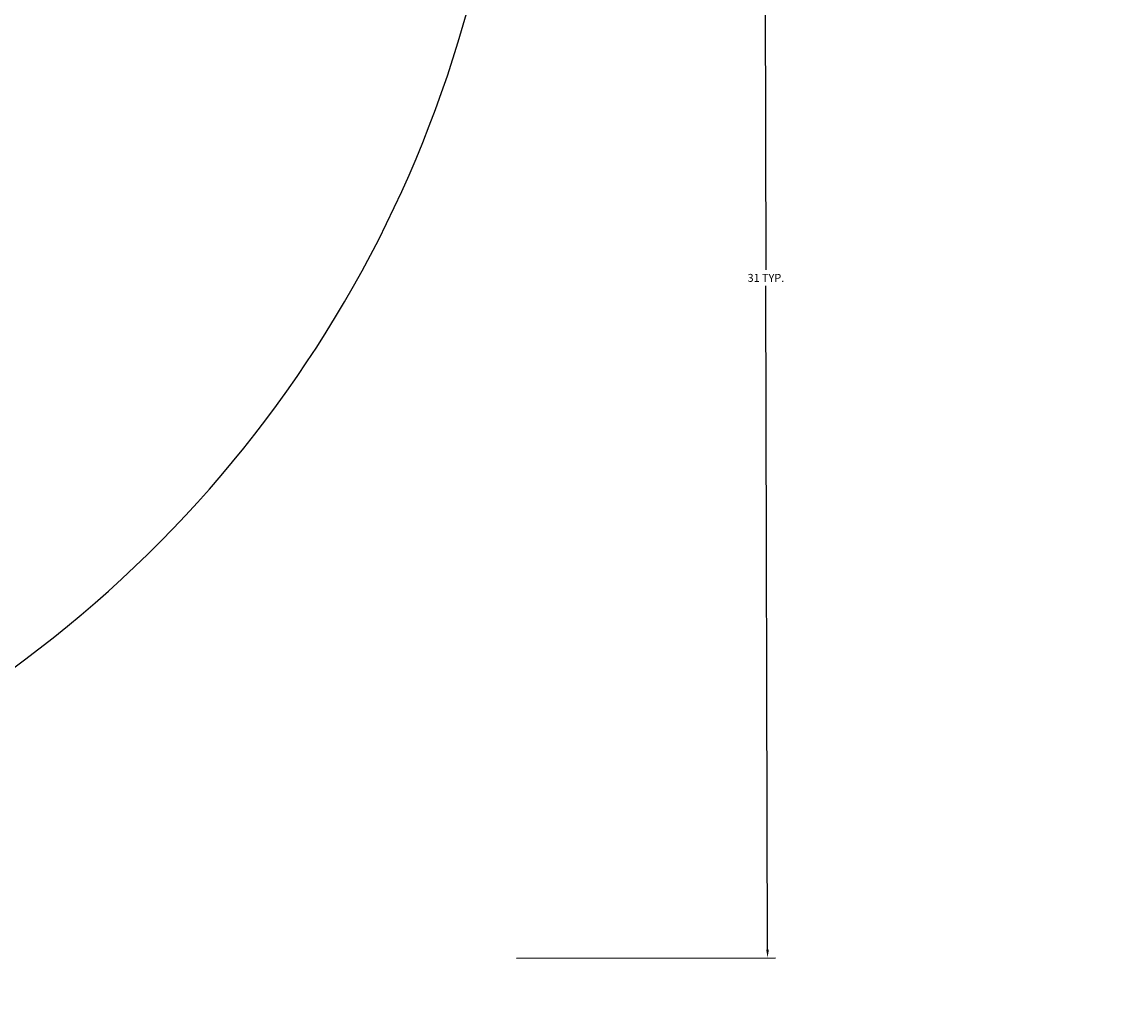
# Model space of a CAD drawing. Units: inches. Extents: x 963 to 2075, y 289 to 2657.
# Tile 10 of 98: x 1399 to 1424, y 1675 to 1696. Entities that reach past the tile are written whole.
import ezdxf

# ---------------------------------------------------------------- set-up
doc = ezdxf.new("R2010")
doc.units = ezdxf.units.IN
for name, color, linetype, lineweight in [('A-ANNO-DIMS', 2, 'Continuous', 18), ('A-DOOR', 4, 'Continuous', 25), ('A-WALL-PATT', 8, 'Continuous', 13)]:
    doc.layers.add(name, color=color, linetype=linetype, lineweight=lineweight)
doc.styles.get("Standard").update_dxf_attribs({"font": 'arial.ttf'})
doc.dimstyles.get("Standard").update_dxf_attribs({"dimtxt": 0.18, "dimasz": 0.18, "dimexe": 0.18, "dimexo": 0.0625, "dimgap": 0.09, "dimtad": 0, "dimtih": 1, "dimtoh": 1, "dimdec": 4, "dimzin": 0, "dimdsep": 46, "dimtxsty": 'Standard', "dimcen": 0.09, "dimadec": 0, "dimazin": 0, "dimtfac": 1, "dimtdec": 4, "dimtofl": 0, "dimtmove": 0, "dimatfit": 3, "dimfxl": 1, "dimtolj": 1, "dimtzin": 0, "dimarcsym": 0})

# ---------------------------------------------------------------- blocks, each defined once
blk = doc.blocks.new('DOOR-5')
blk.add_arc((27.907, 27.321), 27.321, 161.4794, 270)
blk = doc.blocks.new('*D39')
at = {"layer": 'A-ANNO-DIMS', "color": 0, "lineweight": -2, "transparency": 16777216}
for p, q in [((1410.194, 1705.998), (1416.049, 1706.012)), ((1415.869, 1705.832), (1415.906, 1690.845)), ((1415.944, 1675.494), (1415.907, 1690.481)), ((1410.269, 1675.3), (1416.124, 1675.314))]:
    blk.add_line(p, q, dxfattribs=at)
at = {"layer": 'A-ANNO-DIMS', "color": 0, "transparency": 16777216}
for points in [[(1415.899, 1705.832), (1415.839, 1705.832), (1415.869, 1706.012)], [(1415.974, 1675.494), (1415.914, 1675.494), (1415.944, 1675.314)]]:
    blk.add_solid(points, dxfattribs=at)
at = {"layer": 'Defpoints', "color": 0, "transparency": 16777216}
for p in [(1410.131, 1705.998), (1415.869, 1706.012), (1410.207, 1675.299)]:
    blk.add_point(p, dxfattribs=at)
at = {"layer": 'A-ANNO-DIMS', "color": 0, "transparency": 16777216, "insert": (1415.906, 1690.663), "char_height": 0.18, "attachment_point": 5}
blk.add_mtext('\\A1;31 TYP.', dxfattribs=at)

msp = doc.modelspace()

# ---------------------------------------------------------------- hatches: boundary and pattern name
at = {"layer": 'A-WALL-PATT'}
h = msp.add_hatch(dxfattribs=at)
h.set_pattern_fill('ANSI32', color=256)
h.paths.add_polyline_path([(1296.922, 2558.318), (1203.922, 2558.318), (1203.922, 2493.818), (1191.533, 2493.818), (1191.533, 2489.318), (1211.063, 2489.318), (1211.063, 2492.02), (1211.063, 2493.818), (1208.422, 2493.818), (1208.422, 2553.818), (1292.422, 2553.818), (1292.422, 2538.863), (1296.922, 2538.863)])
h.paths.add_polyline_path([(1442.422, 2558.318), (1349.422, 2558.318), (1349.422, 2538.943), (1353.922, 2538.943), (1353.922, 2553.818), (1437.922, 2553.818), (1437.922, 2493.818), (1434.542, 2493.818), (1434.542, 2489.318), (1448.311, 2489.318), (1448.311, 2491.568), (1448.311, 2493.818), (1442.422, 2493.818)])
h.paths.add_polyline_path([(1415.554, 2491.568), (1415.554, 2493.818), (1340.941, 2493.818), (1340.941, 2489.318), (1371.922, 2489.318), (1371.922, 2378.318), (1367.596, 2378.318), (1367.596, 2373.818), (1371.922, 2373.818), (1371.922, 2355.185), (1376.422, 2355.185), (1376.422, 2489.318), (1415.554, 2489.318)])
h.paths.add_polyline_path([(1304.941, 2491.568), (1304.941, 2493.818), (1296.922, 2493.818), (1296.922, 2514.863), (1292.422, 2514.863), (1292.422, 2493.818), (1232.808, 2493.818), (1232.808, 2489.318), (1256.422, 2489.318), (1256.422, 2327.318), (1253.714, 2327.318), (1253.714, 2322.818), (1328.422, 2322.818), (1328.422, 2331.147), (1323.922, 2331.147), (1323.922, 2327.318), (1260.922, 2327.318), (1260.922, 2373.818), (1323.922, 2373.818), (1323.922, 2357.812), (1328.422, 2357.812), (1328.422, 2373.818), (1346.007, 2373.818), (1346.007, 2376.068), (1346.007, 2378.318), (1260.922, 2378.318), (1260.922, 2489.318), (1304.941, 2489.318)])
h.paths.add_polyline_path([(1226.654, 2327.318), (1124.422, 2327.318), (1124.422, 2347.447), (1119.922, 2347.447), (1119.922, 2322.818), (1163.422, 2322.818), (1163.422, 2305.435), (1165.672, 2305.435), (1167.922, 2305.435), (1167.922, 2322.818), (1226.654, 2322.818), (1226.654, 2325.068)])
h.paths.add_polyline_path([(1095.922, 2489.318), (1124.422, 2489.318), (1131.533, 2489.318), (1131.533, 2491.568), (1131.533, 2493.818), (1119.922, 2493.818), (1091.422, 2493.818), (1091.422, 2417.318), (1095.922, 2417.318), (1119.922, 2417.318), (1119.922, 2407.447), (1124.422, 2407.447), (1124.422, 2421.818), (1095.922, 2421.818)])
h.paths.add_polyline_path([(1512.922, 2558.318), (1508.422, 2558.318), (1508.422, 2493.818), (1503.401, 2493.818), (1503.401, 2489.318), (1508.422, 2489.318), (1508.422, 2327.318), (1376.422, 2327.318), (1376.422, 2330.273), (1371.922, 2330.273), (1371.922, 2298.744), (1376.422, 2298.744), (1376.422, 2322.818), (1508.422, 2322.818), (1508.422, 2165.318), (1504.255, 2165.318), (1504.255, 2160.818), (1508.422, 2160.818), (1508.422, 2108.318), (1512.922, 2108.318), (1512.922, 2160.818), (1516.182, 2160.818), (1516.182, 2163.068), (1516.182, 2165.318), (1512.922, 2165.318), (1512.922, 2322.818), (1644.922, 2322.818), (1644.922, 2298.744), (1649.422, 2298.744), (1649.422, 2322.818), (1649.422, 2330.944), (1647.172, 2330.944), (1644.922, 2330.944), (1644.922, 2327.318), (1512.922, 2327.318), (1512.922, 2489.318), (1516.759, 2489.318), (1516.759, 2491.568), (1516.759, 2493.818), (1512.922, 2493.818)])
h.paths.add_polyline_path([(1671.922, 2558.318), (1578.922, 2558.318), (1578.922, 2493.818), (1573.526, 2493.818), (1573.526, 2489.318), (1586.537, 2489.318), (1586.537, 2491.568), (1586.537, 2493.818), (1583.422, 2493.818), (1583.422, 2553.818), (1667.422, 2553.818), (1667.422, 2541.109), (1671.922, 2541.109)])
h.paths.add_polyline_path([(1681.257, 2493.818), (1671.922, 2493.818), (1671.922, 2517.109), (1667.422, 2517.109), (1667.422, 2493.818), (1610.218, 2493.818), (1610.218, 2489.318), (1644.922, 2489.318), (1644.922, 2357.865), (1649.422, 2357.865), (1649.422, 2373.818), (1652.203, 2373.818), (1652.203, 2375.827), (1652.203, 2378.318), (1649.422, 2378.318), (1649.422, 2489.318), (1681.257, 2489.318), (1681.257, 2491.568)])
h.paths.add_polyline_path([(1821.922, 2558.318), (1728.922, 2558.318), (1728.922, 2541), (1733.422, 2541), (1733.422, 2553.818), (1817.422, 2553.818), (1817.422, 2493.818), (1813.507, 2493.818), (1813.507, 2489.318), (1830.078, 2489.318), (1830.078, 2491.568), (1830.078, 2493.818), (1821.922, 2493.818)])
h.paths.add_polyline_path([(1794.244, 2493.818), (1717.257, 2493.818), (1717.257, 2489.318), (1760.422, 2489.318), (1760.422, 2378.318), (1674.401, 2378.318), (1674.401, 2373.818), (1692.922, 2373.818), (1692.922, 2356.954), (1697.422, 2356.954), (1697.422, 2373.818), (1760.422, 2373.818), (1760.422, 2327.318), (1697.422, 2327.318), (1697.422, 2333.341), (1692.922, 2333.341), (1692.922, 2322.818), (1768.037, 2322.818), (1768.037, 2325.068), (1768.037, 2327.318), (1764.922, 2327.318), (1764.922, 2489.318), (1794.244, 2489.318)])
h.paths.add_polyline_path([(1733.422, 2517), (1728.922, 2517), (1728.922, 2493.818), (1733.422, 2493.818)], flags=17)
h.paths.add_polyline_path([(1929.922, 2493.818), (1890.078, 2493.818), (1890.078, 2489.318), (1896.922, 2489.318), (1925.422, 2489.318), (1925.422, 2421.818), (1896.922, 2421.818), (1896.922, 2408.318), (1901.422, 2408.318), (1901.422, 2417.318), (1925.422, 2417.318), (1929.922, 2417.318)])
h.paths.add_polyline_path([(1901.422, 2348.318), (1896.922, 2348.318), (1896.922, 2327.318), (1800.423, 2327.318), (1800.423, 2322.818), (1853.422, 2322.818), (1853.422, 2309.453), (1857.922, 2309.453), (1857.922, 2322.818), (1901.422, 2322.818)])
h.paths.add_polyline_path([(1857.922, 2249.453), (1853.422, 2249.453), (1853.422, 2214.818), (1686.309, 2214.818), (1686.309, 2210.318), (1853.422, 2210.318), (1853.422, 2202.134), (1857.922, 2202.134), (1857.922, 2210.318)])
h.paths.add_polyline_path([(1857.922, 2142.134), (1853.422, 2142.134), (1853.422, 2115.422), (1841.422, 2115.422), (1841.422, 2088.531), (1841.422, 2046.949), (1845.922, 2046.949), (1845.922, 2110.922), (1905.922, 2110.922), (1905.922, 2092.517), (1910.422, 2092.517), (1910.422, 2115.422), (1857.922, 2115.422)])
h.paths.add_polyline_path([(1532.436, 1482.342), (1573.456, 1482.342), (1573.456, 1501), (1532.436, 1501)], flags=9)
h.paths.add_polyline_path([(1438.658, 1486.302), (1479.678, 1486.302), (1479.678, 1504.96), (1438.658, 1504.96)], flags=9)
h.paths.add_polyline_path([(1411.215, 1365.308), (1659.139, 1365.308), (1659.139, 1402.401), (1411.215, 1402.401)], flags=9)
h.paths.add_polyline_path([(1185.671, 2296.298), (1248.16, 2296.298), (1248.16, 2314.955), (1185.671, 2314.955)], flags=9)
h.paths.add_polyline_path([(1177.31, 2187.35), (1216.15, 2187.35), (1216.15, 2206.007), (1177.31, 2206.007)], flags=9)
h.paths.add_polyline_path([(1295.101, 1602.083), (1328.26, 1602.083), (1328.26, 1620.741), (1295.101, 1620.741)], flags=9)
h.paths.add_polyline_path([(1525.126, 2005.99), (1558.39, 2005.99), (1558.39, 2024.648), (1525.126, 2024.648)], flags=9)
h.paths.add_polyline_path([(1459.606, 1977.125), (1472.195, 1977.125), (1472.195, 1987.429), (1459.606, 1987.429)], flags=9)
h.paths.add_polyline_path([(1467.815, 2053.676), (1480.018, 2053.676), (1480.018, 2063.979), (1467.815, 2063.979)], flags=9)
h.paths.add_polyline_path([(1555.184, 2119.02), (1584.563, 2119.02), (1584.563, 2137.678), (1555.184, 2137.678)], flags=25)
h.paths.add_polyline_path([(1405.389, 2115.291), (1444.478, 2115.291), (1444.478, 2133.948), (1405.389, 2133.948)], flags=25)
h.paths.add_polyline_path([(1698.482, 2004.259), (1727.695, 2004.259), (1727.695, 2022.916), (1698.482, 2022.916)], flags=9)
h.paths.add_polyline_path([(1612.158, 1972.855), (1629.016, 1972.855), (1629.016, 1983.159), (1612.158, 1983.159)], flags=9)
h.paths.add_polyline_path([(1608.289, 2060.036), (1625.147, 2060.036), (1625.147, 2070.34), (1608.289, 2070.34)], flags=9)
h.paths.add_polyline_path([(1527.954, 1684.402), (1566.795, 1684.402), (1566.795, 1703.06), (1527.954, 1703.06)], flags=9)
h.paths.add_polyline_path([(1422.792, 1683.59), (1461.633, 1683.59), (1461.633, 1702.247), (1422.792, 1702.247)], flags=9)
h.paths.add_polyline_path([(1531.262, 1732.459), (1574.015, 1732.459), (1574.015, 1751.116), (1531.262, 1751.116)], flags=9)
h.paths.add_polyline_path([(1402.872, 1732.845), (1439.799, 1732.845), (1439.799, 1751.502), (1402.872, 1751.502)], flags=9)
h.paths.add_polyline_path([(1243.122, 1923.132), (1281.962, 1923.132), (1281.962, 1941.79), (1243.122, 1941.79)], flags=9)
h.paths.add_polyline_path([(1181.752, 1792.268), (1244.241, 1792.268), (1244.241, 1810.926), (1181.752, 1810.926)], flags=9)
h.paths.add_polyline_path([(1265.822, 1670.3), (1316.071, 1670.3), (1316.071, 1688.957), (1265.822, 1688.957)], flags=9)
h.paths.add_polyline_path([(1140.263, 1676.054), (1179.104, 1676.054), (1179.104, 1694.711), (1140.263, 1694.711)], flags=9)
h.paths.add_polyline_path([(1107.49, 1490.889), (1143.374, 1490.889), (1143.374, 1509.546), (1107.49, 1509.546)], flags=9)
h.paths.add_polyline_path([(1217.584, 1483.899), (1246.741, 1483.899), (1246.741, 1502.556), (1217.584, 1502.556)], flags=9)
h.paths.add_polyline_path([(1389.21, 1486.919), (1418.367, 1486.919), (1418.367, 1505.576), (1389.21, 1505.576)], flags=9)
h.paths.add_polyline_path([(1672.208, 1602.083), (1705.366, 1602.083), (1705.366, 1620.741), (1672.208, 1620.741)], flags=9)
h.paths.add_polyline_path([(1752.082, 1522.638), (1781.24, 1522.638), (1781.24, 1541.295), (1752.082, 1541.295)], flags=9)
h.paths.add_polyline_path([(1848.275, 1491.26), (1884.158, 1491.26), (1884.158, 1509.918), (1848.275, 1509.918)], flags=9)
h.paths.add_polyline_path([(1822.47, 1685.62), (1861.31, 1685.62), (1861.31, 1704.278), (1822.47, 1704.278)], flags=9)
h.paths.add_polyline_path([(1713.195, 1672.232), (1763.444, 1672.232), (1763.444, 1690.889), (1713.195, 1690.889)], flags=9)
h.paths.add_polyline_path([(1736.619, 1790.578), (1799.109, 1790.578), (1799.109, 1809.235), (1736.619, 1809.235)], flags=9)
h.paths.add_polyline_path([(1691.491, 1916.355), (1730.332, 1916.355), (1730.332, 1935.013), (1691.491, 1935.013)], flags=9)
h.paths.add_polyline_path([(1764.872, 1973.922), (1794.306, 1973.922), (1794.306, 1992.58), (1764.872, 1992.58)], flags=9)
h.paths.add_polyline_path([(1767.854, 2034.017), (1797.288, 2034.017), (1797.288, 2052.674), (1767.854, 2052.674)], flags=9)
h.paths.add_polyline_path([(1851.593, 2060.331), (1880.751, 2060.331), (1880.751, 2078.989), (1851.593, 2078.989)], flags=25)
h.paths.add_polyline_path([(1688.491, 2086.874), (1727.332, 2086.874), (1727.332, 2105.531), (1688.491, 2105.531)], flags=9)
h.paths.add_polyline_path([(1537.743, 2293.581), (1580.495, 2293.581), (1580.495, 2312.239), (1537.743, 2312.239)], flags=25)
h.paths.add_polyline_path([(1425.587, 2296.109), (1468.34, 2296.109), (1468.34, 2314.766), (1425.587, 2314.766)], flags=25)
h.paths.add_polyline_path([(1278.518, 2004.184), (1307.72, 2004.184), (1307.72, 2022.841), (1278.518, 2022.841)], flags=9)
h.paths.add_polyline_path([(1193.282, 1973.635), (1222.715, 1973.635), (1222.715, 1992.292), (1193.282, 1992.292)], flags=9)
h.paths.add_polyline_path([(1192.411, 2040.577), (1221.845, 2040.577), (1221.845, 2059.234), (1192.411, 2059.234)], flags=9)
h.paths.add_polyline_path([(1130.603, 1951.393), (1159.76, 1951.393), (1159.76, 1970.05), (1130.603, 1970.05)], flags=9)
h.paths.add_polyline_path([(1132.827, 2052.494), (1161.984, 2052.494), (1161.984, 2071.151), (1132.827, 2071.151)], flags=9)
h.paths.add_polyline_path([(1265.128, 2334.619), (1315.377, 2334.619), (1315.377, 2353.277), (1265.128, 2353.277)], flags=25)
h.paths.add_polyline_path([(1136.741, 2330.785), (1175.582, 2330.785), (1175.582, 2349.443), (1136.741, 2349.443)], flags=9)
h.paths.add_polyline_path([(1287.422, 2417.204), (1320.58, 2417.204), (1320.58, 2435.861), (1287.422, 2435.861)], flags=25)
h.paths.add_polyline_path([(1430.988, 2329.159), (1469.828, 2329.159), (1469.828, 2347.816), (1430.988, 2347.816)], flags=25)
h.paths.add_polyline_path([(1525.424, 2329.213), (1564.264, 2329.213), (1564.264, 2347.87), (1525.424, 2347.87)], flags=25)
h.paths.add_polyline_path([(1684.525, 2382.799), (1717.683, 2382.799), (1717.683, 2401.457), (1684.525, 2401.457)], flags=25)
h.paths.add_polyline_path([(1704.805, 2340.293), (1755.054, 2340.293), (1755.054, 2358.95), (1704.805, 2358.95)], flags=25)
h.paths.add_polyline_path([(1694.113, 2287.757), (1756.602, 2287.757), (1756.602, 2306.414), (1694.113, 2306.414)], flags=9)
h.paths.add_polyline_path([(1815.778, 2329.861), (1854.618, 2329.861), (1854.618, 2348.518), (1815.778, 2348.518)], flags=9)
h.paths.add_polyline_path([(1842.873, 2514.256), (1878.756, 2514.256), (1878.756, 2532.914), (1842.873, 2532.914)], flags=9)
h.paths.add_polyline_path([(1769.513, 2531.447), (1798.671, 2531.447), (1798.671, 2550.104), (1769.513, 2550.104)], flags=25)
h.paths.add_polyline_path([(1594.772, 2518.468), (1623.93, 2518.468), (1623.93, 2537.125), (1594.772, 2537.125)], flags=25)
h.paths.add_polyline_path([(1520.723, 2516.185), (1556.606, 2516.185), (1556.606, 2534.842), (1520.723, 2534.842)], flags=25)
h.paths.add_polyline_path([(1464.456, 2516.694), (1500.34, 2516.694), (1500.34, 2535.351), (1464.456, 2535.351)], flags=25)
h.paths.add_polyline_path([(1365.696, 2528.97), (1394.854, 2528.97), (1394.854, 2547.627), (1365.696, 2547.627)], flags=25)
h.paths.add_polyline_path([(1222.838, 2516.231), (1251.995, 2516.231), (1251.995, 2534.889), (1222.838, 2534.889)], flags=25)
h.paths.add_polyline_path([(1104.545, 2509.6), (1140.429, 2509.6), (1140.429, 2528.257), (1104.545, 2528.257)], flags=9)
h = msp.add_hatch(dxfattribs=at)
h.set_pattern_fill('ANSI32', color=256)
h.paths.add_polyline_path([(1335.968, 2212.568), (1335.968, 2214.818), (1167.922, 2214.818), (1167.922, 2245.435), (1163.422, 2245.435), (1163.422, 2210.318), (1163.422, 2194.812), (1167.922, 2194.812), (1167.922, 2210.318), (1335.968, 2210.318)])
h.paths.add_polyline_path([(1532.436, 1482.342), (1573.456, 1482.342), (1573.456, 1501), (1532.436, 1501)], flags=9)
h.paths.add_polyline_path([(1438.658, 1486.302), (1479.678, 1486.302), (1479.678, 1504.96), (1438.658, 1504.96)], flags=9)
h.paths.add_polyline_path([(1411.215, 1365.308), (1659.139, 1365.308), (1659.139, 1402.401), (1411.215, 1402.401)], flags=9)
h.paths.add_polyline_path([(1185.671, 2296.298), (1248.16, 2296.298), (1248.16, 2314.955), (1185.671, 2314.955)], flags=9)
h.paths.add_polyline_path([(1177.31, 2187.35), (1216.15, 2187.35), (1216.15, 2206.007), (1177.31, 2206.007)], flags=9)
h.paths.add_polyline_path([(1295.101, 1602.083), (1328.26, 1602.083), (1328.26, 1620.741), (1295.101, 1620.741)], flags=9)
h.paths.add_polyline_path([(1525.126, 2005.99), (1558.39, 2005.99), (1558.39, 2024.648), (1525.126, 2024.648)], flags=9)
h.paths.add_polyline_path([(1459.606, 1977.125), (1472.195, 1977.125), (1472.195, 1987.429), (1459.606, 1987.429)], flags=9)
h.paths.add_polyline_path([(1467.815, 2053.676), (1480.018, 2053.676), (1480.018, 2063.979), (1467.815, 2063.979)], flags=9)
h.paths.add_polyline_path([(1555.184, 2119.02), (1584.563, 2119.02), (1584.563, 2137.678), (1555.184, 2137.678)], flags=9)
h.paths.add_polyline_path([(1405.389, 2115.291), (1444.478, 2115.291), (1444.478, 2133.948), (1405.389, 2133.948)], flags=9)
h.paths.add_polyline_path([(1698.482, 2004.259), (1727.695, 2004.259), (1727.695, 2022.916), (1698.482, 2022.916)], flags=9)
h.paths.add_polyline_path([(1612.158, 1972.855), (1629.016, 1972.855), (1629.016, 1983.159), (1612.158, 1983.159)], flags=9)
h.paths.add_polyline_path([(1608.289, 2060.036), (1625.147, 2060.036), (1625.147, 2070.34), (1608.289, 2070.34)], flags=9)
h.paths.add_polyline_path([(1527.954, 1684.402), (1566.795, 1684.402), (1566.795, 1703.06), (1527.954, 1703.06)], flags=9)
h.paths.add_polyline_path([(1422.792, 1683.59), (1461.633, 1683.59), (1461.633, 1702.247), (1422.792, 1702.247)], flags=9)
h.paths.add_polyline_path([(1531.262, 1732.459), (1574.015, 1732.459), (1574.015, 1751.116), (1531.262, 1751.116)], flags=9)
h.paths.add_polyline_path([(1402.872, 1732.845), (1439.799, 1732.845), (1439.799, 1751.502), (1402.872, 1751.502)], flags=9)
h.paths.add_polyline_path([(1243.122, 1923.132), (1281.962, 1923.132), (1281.962, 1941.79), (1243.122, 1941.79)], flags=9)
h.paths.add_polyline_path([(1181.752, 1792.268), (1244.241, 1792.268), (1244.241, 1810.926), (1181.752, 1810.926)], flags=9)
h.paths.add_polyline_path([(1265.822, 1670.3), (1316.071, 1670.3), (1316.071, 1688.957), (1265.822, 1688.957)], flags=9)
h.paths.add_polyline_path([(1140.263, 1676.054), (1179.104, 1676.054), (1179.104, 1694.711), (1140.263, 1694.711)], flags=9)
h.paths.add_polyline_path([(1107.49, 1490.889), (1143.374, 1490.889), (1143.374, 1509.546), (1107.49, 1509.546)], flags=9)
h.paths.add_polyline_path([(1217.584, 1483.899), (1246.741, 1483.899), (1246.741, 1502.556), (1217.584, 1502.556)], flags=9)
h.paths.add_polyline_path([(1389.21, 1486.919), (1418.367, 1486.919), (1418.367, 1505.576), (1389.21, 1505.576)], flags=9)
h.paths.add_polyline_path([(1672.208, 1602.083), (1705.366, 1602.083), (1705.366, 1620.741), (1672.208, 1620.741)], flags=9)
h.paths.add_polyline_path([(1752.082, 1522.638), (1781.24, 1522.638), (1781.24, 1541.295), (1752.082, 1541.295)], flags=9)
h.paths.add_polyline_path([(1848.275, 1491.26), (1884.158, 1491.26), (1884.158, 1509.918), (1848.275, 1509.918)], flags=9)
h.paths.add_polyline_path([(1822.47, 1685.62), (1861.31, 1685.62), (1861.31, 1704.278), (1822.47, 1704.278)], flags=9)
h.paths.add_polyline_path([(1713.195, 1672.232), (1763.444, 1672.232), (1763.444, 1690.889), (1713.195, 1690.889)], flags=9)
h.paths.add_polyline_path([(1736.619, 1790.578), (1799.109, 1790.578), (1799.109, 1809.235), (1736.619, 1809.235)], flags=9)
h.paths.add_polyline_path([(1691.491, 1916.355), (1730.332, 1916.355), (1730.332, 1935.013), (1691.491, 1935.013)], flags=9)
h.paths.add_polyline_path([(1764.872, 1973.922), (1794.306, 1973.922), (1794.306, 1992.58), (1764.872, 1992.58)], flags=9)
h.paths.add_polyline_path([(1767.854, 2034.017), (1797.288, 2034.017), (1797.288, 2052.674), (1767.854, 2052.674)], flags=9)
h.paths.add_polyline_path([(1851.593, 2060.331), (1880.751, 2060.331), (1880.751, 2078.989), (1851.593, 2078.989)], flags=9)
h.paths.add_polyline_path([(1688.491, 2086.874), (1727.332, 2086.874), (1727.332, 2105.531), (1688.491, 2105.531)], flags=9)
h.paths.add_polyline_path([(1537.743, 2293.581), (1580.495, 2293.581), (1580.495, 2312.239), (1537.743, 2312.239)], flags=9)
h.paths.add_polyline_path([(1425.587, 2296.109), (1468.34, 2296.109), (1468.34, 2314.766), (1425.587, 2314.766)], flags=9)
h.paths.add_polyline_path([(1278.518, 2004.184), (1307.72, 2004.184), (1307.72, 2022.841), (1278.518, 2022.841)], flags=9)
h.paths.add_polyline_path([(1193.282, 1973.635), (1222.715, 1973.635), (1222.715, 1992.292), (1193.282, 1992.292)], flags=9)
h.paths.add_polyline_path([(1192.411, 2040.577), (1221.845, 2040.577), (1221.845, 2059.234), (1192.411, 2059.234)], flags=9)
h.paths.add_polyline_path([(1130.603, 1951.393), (1159.76, 1951.393), (1159.76, 1970.05), (1130.603, 1970.05)], flags=9)
h.paths.add_polyline_path([(1132.827, 2052.494), (1161.984, 2052.494), (1161.984, 2071.151), (1132.827, 2071.151)], flags=9)
h.paths.add_polyline_path([(1265.128, 2334.619), (1315.377, 2334.619), (1315.377, 2353.277), (1265.128, 2353.277)], flags=9)
h.paths.add_polyline_path([(1136.741, 2330.785), (1175.582, 2330.785), (1175.582, 2349.443), (1136.741, 2349.443)], flags=9)
h.paths.add_polyline_path([(1287.422, 2417.204), (1320.58, 2417.204), (1320.58, 2435.861), (1287.422, 2435.861)], flags=9)
h.paths.add_polyline_path([(1430.988, 2329.159), (1469.828, 2329.159), (1469.828, 2347.816), (1430.988, 2347.816)], flags=9)
h.paths.add_polyline_path([(1525.424, 2329.213), (1564.264, 2329.213), (1564.264, 2347.87), (1525.424, 2347.87)], flags=9)
h.paths.add_polyline_path([(1684.525, 2382.799), (1717.683, 2382.799), (1717.683, 2401.457), (1684.525, 2401.457)], flags=9)
h.paths.add_polyline_path([(1704.805, 2340.293), (1755.054, 2340.293), (1755.054, 2358.95), (1704.805, 2358.95)], flags=9)
h.paths.add_polyline_path([(1694.113, 2287.757), (1756.602, 2287.757), (1756.602, 2306.414), (1694.113, 2306.414)], flags=9)
h.paths.add_polyline_path([(1815.778, 2329.861), (1854.618, 2329.861), (1854.618, 2348.518), (1815.778, 2348.518)], flags=9)
h.paths.add_polyline_path([(1842.873, 2514.256), (1878.756, 2514.256), (1878.756, 2532.914), (1842.873, 2532.914)], flags=9)
h.paths.add_polyline_path([(1769.513, 2531.447), (1798.671, 2531.447), (1798.671, 2550.104), (1769.513, 2550.104)], flags=9)
h.paths.add_polyline_path([(1594.772, 2518.468), (1623.93, 2518.468), (1623.93, 2537.125), (1594.772, 2537.125)], flags=9)
h.paths.add_polyline_path([(1520.723, 2516.185), (1556.606, 2516.185), (1556.606, 2534.842), (1520.723, 2534.842)], flags=9)
h.paths.add_polyline_path([(1464.456, 2516.694), (1500.34, 2516.694), (1500.34, 2535.351), (1464.456, 2535.351)], flags=9)
h.paths.add_polyline_path([(1365.696, 2528.97), (1394.854, 2528.97), (1394.854, 2547.627), (1365.696, 2547.627)], flags=9)
h.paths.add_polyline_path([(1222.838, 2516.231), (1251.995, 2516.231), (1251.995, 2534.889), (1222.838, 2534.889)], flags=9)
h.paths.add_polyline_path([(1104.545, 2509.6), (1140.429, 2509.6), (1140.429, 2528.257), (1104.545, 2528.257)], flags=9)

# ---------------------------------------------------------------- block references
at = {"layer": 'A-DOOR', "rotation": 90.14142652708767}
msp.add_blockref('DOOR-5', (1410.204, 1676.091), dxfattribs=at)

# ---------------------------------------------------------------- dimensions: what is measured, and where the dimension line sits
at = {"layer": 'A-ANNO-DIMS'}
dim = msp.add_linear_dim(base=(1415.869, 1706.012), p1=(1410.207, 1675.299), p2=(1410.131, 1705.998), angle=90.1414, text='<> TYP.', dimstyle='Standard', override={"dimdec": 0, "dimlfac": 1, "dimrnd": 0, "dimzin": 0, "dimdsep": 46, "dimlunit": 2}, dxfattribs=at)
dim.commit()
dim.dimension.update_dxf_attribs({"geometry": '*D39', "text_midpoint": (1415.906, 1690.663)})

doc.saveas('drawing.dxf')
